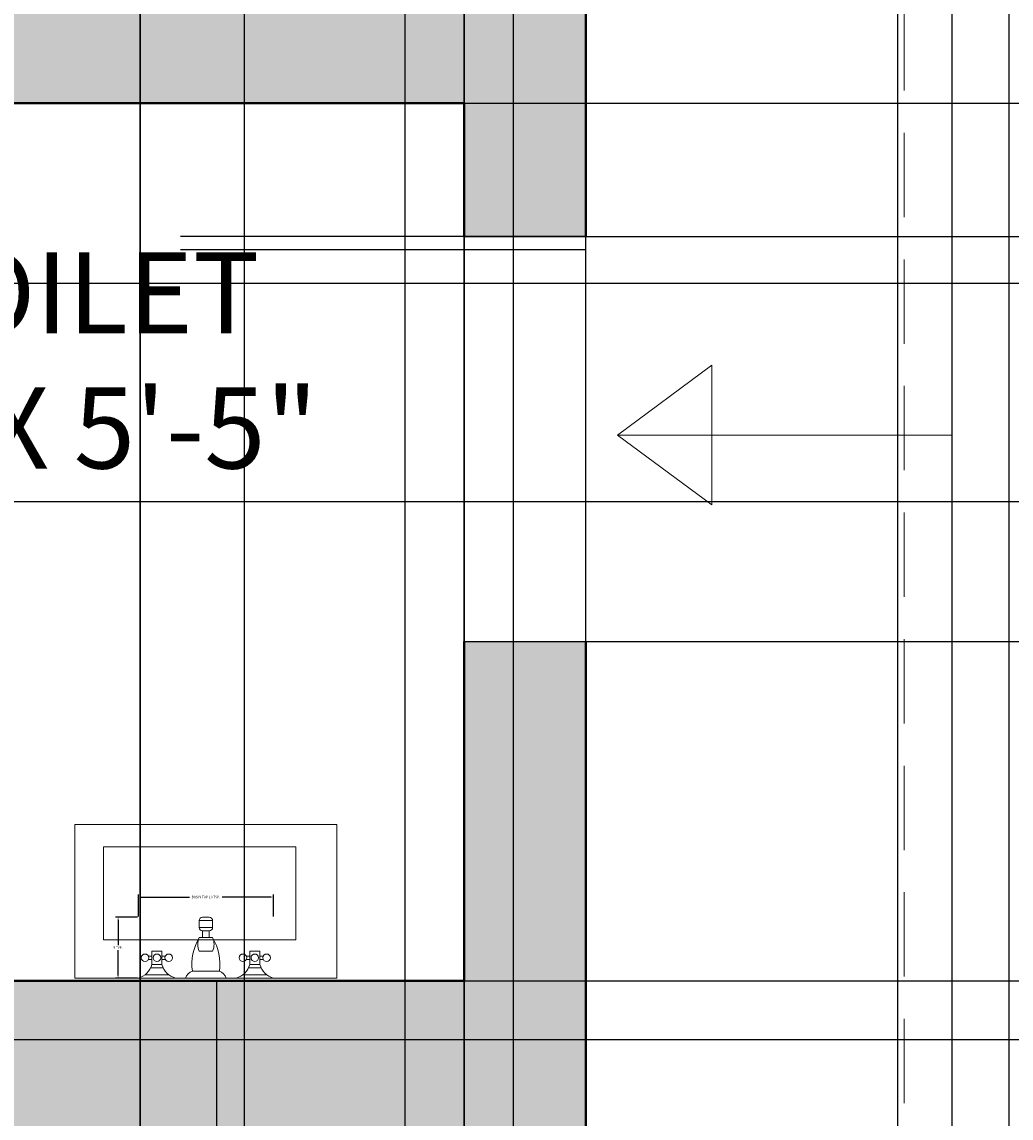
# Model space of a CAD drawing. Units: inches. Extents: x 818 to 1898, y 976 to 2364.
# Tile 55 of 96: x 1673 to 1746, y 1792 to 1873. Entities that reach past the tile are written whole.
import ezdxf

# ---------------------------------------------------------------- set-up
doc = ezdxf.new("R2010")
doc.units = ezdxf.units.IN
doc.header["$LTSCALE"] = 5
doc.header["$MEASUREMENT"] = 0
doc.linetypes.add('HIDDEN', pattern=[0.375, 0.25, -0.125])
for name, color, linetype, lineweight in [('A-ANNO-DIMS', 2, 'Continuous', 18), ('A-ANNO-SYMB', 7, 'Continuous', 18), ('A-AREA-IDEN', 7, 'Continuous', 18), ('A-DOOR', 3, 'Continuous', 25), ('A-FLOR-FIXT', 9, 'Continuous', 18), ('A-FLOR-OVHD', 8, 'HIDDEN', 13), ('A-FLOR-STRS', 7, 'Continuous', 25), ('A-WALL', 7, 'Continuous', 40)]:
    doc.layers.add(name, color=color, linetype=linetype, lineweight=lineweight)
doc.layers.add('A-WALL-PATT', color=251, linetype='Continuous', lineweight=13, true_color=0x636466)
doc.styles.get("Standard").update_dxf_attribs({"font": 'arial.ttf'})
doc.dimstyles.get("Standard").update_dxf_attribs({"dimtxt": 0.18, "dimasz": 0.18, "dimexe": 0.18, "dimexo": 0.0625, "dimgap": 0.09, "dimtad": 0, "dimtih": 1, "dimtoh": 1, "dimdec": 4, "dimzin": 0, "dimdsep": 46, "dimtxsty": 'Standard', "dimcen": 0.09, "dimadec": 0, "dimazin": 0, "dimtfac": 1, "dimtdec": 4, "dimtofl": 0, "dimtmove": 0, "dimatfit": 3, "dimfxl": 1, "dimtolj": 1, "dimtzin": 0, "dimarcsym": 0})

# ---------------------------------------------------------------- blocks, each defined once
blk = doc.blocks.new('Faucet - Bathroom front')
for p, q in [((-0.5, 4.25), (0.5, 4.25)), ((0.5, 3.75), (-0.5, 3.75)), ((-0.25, 3), (-0.25, 3.5)), ((0.25, 3.5), (0.25, 3)), ((-0.5, 3), (0.5, 3)), ((-4, 1.625), (-4.25, 1.625)), ((-3.25, 1.625), (-3, 1.625)), ((0.5, 2), (-0.5, 2)), ((3.25, 1.625), (3, 1.625)), ((4, 1.625), (4.25, 1.625)), ((-4, 1.375), (-4.25, 1.375)), ((-3.25, 1.375), (-3, 1.375)), ((3.25, 1.375), (3, 1.375)), ((4, 1.375), (4.25, 1.375)), ((-5, 0), (-2.25, 0)), ((-4.5087, 0.25), (-2.7408, 0.25)), ((-3.1442, 0.75), (-4.0979, 0.75)), ((-1.5, 0), (1.5, 0)), ((-1, 0.5), (1, 0.5)), ((2.25, 0), (5, 0)), ((2.7413, 0.25), (4.5092, 0.25)), ((4.1058, 0.75), (3.1521, 0.75))]:
    blk.add_line(p, q)
for points in [[(-0.5, 3.75), (-0.5, 4.25)], [(-0.25, 4.5), (0.25, 4.5)], [(0.5, 4.25), (0.5, 3.75)], [(0.25, 3.5), (-0.25, 3.5)]]:
    blk.add_lwpolyline(points)
for points in [[(-4, 1), (-4, 2), (-3.25, 2), (-3.25, 1)], [(3.25, 1), (3.25, 2), (4, 2), (4, 1)]]:
    blk.add_lwpolyline(points, close=True)
for centre in [(-4.5, 1.5), (-3.625, 1.5), (-2.75, 1.5), (2.75, 1.5), (3.625, 1.5), (4.5, 1.5)]:
    blk.add_circle(centre, 0.2795)
for centre, radius, start, end in [((-0.2575, 4.2575), 0.2426, 88.22243, 181.7776), ((0.2575, 4.2575), 0.2426, 358.2224, 91.77757), ((-0.2575, 3.7425), 0.2426, 178.2224, 271.7776), ((0.2575, 3.7425), 0.2426, 268.2224, 1.777565), ((3, 1), 4.0311, 150.2551, 187.125), ((0.6413, 2.5), 1.246, 156.3417, 203.6583), ((-3, 1), 4.0311, 352.875, 29.74488), ((-0.6413, 2.5), 1.246, 336.3417, 23.65835), ((-5.375, 1.375), 1.4252, 285.2551, 344.7449), ((-1.875, 1.375), 1.4252, 195.2551, 254.7449), ((1.875, 1.375), 1.4252, 285.2551, 344.7449), ((5.375, 1.375), 1.4252, 195.2551, 254.7449), ((-0.7962, -0.2038), 0.7327, 106.1502, 163.8498), ((0.7962, -0.2038), 0.7327, 16.1502, 73.84979)]:
    blk.add_arc(centre, radius, start, end)
blk = doc.blocks.new('BASIN-COMPACT')
for points in [[(19.386, 0), (19.386, 11.383), (0, 11.383), (0, 0)], [(16.353, 2.839), (16.353, 9.718), (2.106, 9.718), (2.106, 2.839)]]:
    blk.add_lwpolyline(points, close=True)
blk = doc.blocks.new('ARROW-STEP-UP')
at = {"ltscale": 5}
for p, q in [((0, 5.169), (6.971, 10.338)), ((6.971, 10.338), (6.971, 5.169)), ((24.755, 5.169), (0, 5.169)), ((0, 5.169), (6.971, 0)), ((6.971, 0), (6.971, 5.169))]:
    blk.add_line(p, q, dxfattribs=at)
blk = doc.blocks.new('*D34')
at = {"layer": 'A-ANNO-DIMS', "color": 0, "lineweight": -2, "ltscale": 5, "transparency": 16777216}
for p, q in [((1681.598, 1806.847), (1681.598, 1808.464)), ((1681.778, 1808.284), (1685.382, 1808.284)), ((1691.418, 1808.284), (1687.814, 1808.284)), ((1691.598, 1806.847), (1691.598, 1808.464))]:
    blk.add_line(p, q, dxfattribs=at)
at = {"layer": 'A-ANNO-DIMS', "color": 0, "ltscale": 5, "transparency": 16777216}
for points in [[(1681.778, 1808.314), (1681.778, 1808.254), (1681.598, 1808.284)], [(1691.418, 1808.314), (1691.418, 1808.254), (1691.598, 1808.284)]]:
    blk.add_solid(points, dxfattribs=at)
at = {"layer": 'Defpoints', "color": 0, "ltscale": 5, "transparency": 16777216}
for p in [(1691.598, 1808.284), (1681.598, 1806.784), (1691.598, 1806.784)]:
    blk.add_point(p, dxfattribs=at)
at = {"layer": 'A-ANNO-DIMS', "color": 0, "ltscale": 5, "transparency": 16777216, "insert": (1686.598, 1808.284), "char_height": 0.18, "attachment_point": 5}
blk.add_mtext('\\A1;BASIN TAP 10 TYP.', dxfattribs=at)
blk = doc.blocks.new('*D35')
at = {"layer": 'A-ANNO-DIMS', "color": 0, "lineweight": -2, "ltscale": 5, "transparency": 16777216}
for p, q in [((1681.535, 1806.784), (1679.918, 1806.784)), ((1680.098, 1806.604), (1680.098, 1804.715)), ((1680.098, 1802.462), (1680.098, 1804.352)), ((1681.535, 1802.282), (1679.918, 1802.282))]:
    blk.add_line(p, q, dxfattribs=at)
at = {"layer": 'A-ANNO-DIMS', "color": 0, "ltscale": 5, "transparency": 16777216}
for points in [[(1680.068, 1806.604), (1680.128, 1806.604), (1680.098, 1806.784)], [(1680.068, 1802.462), (1680.128, 1802.462), (1680.098, 1802.282)]]:
    blk.add_solid(points, dxfattribs=at)
at = {"layer": 'Defpoints', "color": 0, "ltscale": 5, "transparency": 16777216}
for p in [(1680.098, 1806.784), (1681.598, 1806.784), (1681.598, 1802.282)]:
    blk.add_point(p, dxfattribs=at)
at = {"layer": 'A-ANNO-DIMS', "color": 0, "ltscale": 5, "transparency": 16777216, "insert": (1680.098, 1804.533), "char_height": 0.18, "attachment_point": 5}
blk.add_mtext('\\A1;5 TYP.', dxfattribs=at)
blk = doc.blocks.new('*D71')
at = {"layer": 'A-ANNO-DIMS', "color": 0, "lineweight": -2, "ltscale": 5, "transparency": 16777216}
for p, q in [((1714.788, 2053.078), (1897.916, 2053.078)), ((1897.736, 2052.898), (1897.736, 1699.76)), ((1897.736, 1346.258), (1897.736, 1699.396)), ((1714.788, 1346.078), (1897.916, 1346.078))]:
    blk.add_line(p, q, dxfattribs=at)
at = {"layer": 'A-ANNO-DIMS', "color": 0, "ltscale": 5, "transparency": 16777216}
for points in [[(1897.706, 2052.898), (1897.766, 2052.898), (1897.736, 2053.078)], [(1897.706, 1346.258), (1897.766, 1346.258), (1897.736, 1346.078)]]:
    blk.add_solid(points, dxfattribs=at)
at = {"layer": 'Defpoints', "color": 0, "ltscale": 5, "transparency": 16777216}
for p in [(1714.725, 2053.078), (1897.736, 2053.078), (1714.725, 1346.078)]:
    blk.add_point(p, dxfattribs=at)
at = {"layer": 'A-ANNO-DIMS', "color": 0, "ltscale": 5, "transparency": 16777216, "insert": (1897.736, 1699.578), "char_height": 0.18, "attachment_point": 5}
blk.add_mtext('\\A1;707', dxfattribs=at)
blk = doc.blocks.new('*D76')
at = {"layer": 'A-ANNO-DIMS', "color": 0, "lineweight": -2, "ltscale": 5, "transparency": 16777216}
for p, q in [((1705.788, 1857.212), (1897.916, 1857.212)), ((1897.736, 1857.032), (1897.736, 1842.394)), ((1897.736, 1827.392), (1897.736, 1842.031)), ((1705.788, 1827.212), (1897.916, 1827.212))]:
    blk.add_line(p, q, dxfattribs=at)
at = {"layer": 'A-ANNO-DIMS', "color": 0, "ltscale": 5, "transparency": 16777216}
for points in [[(1897.706, 1857.032), (1897.766, 1857.032), (1897.736, 1857.212)], [(1897.706, 1827.392), (1897.766, 1827.392), (1897.736, 1827.212)]]:
    blk.add_solid(points, dxfattribs=at)
at = {"layer": 'Defpoints', "color": 0, "ltscale": 5, "transparency": 16777216}
for p in [(1705.725, 1857.212), (1897.736, 1857.212), (1705.725, 1827.212)]:
    blk.add_point(p, dxfattribs=at)
at = {"layer": 'A-ANNO-DIMS', "color": 0, "ltscale": 5, "transparency": 16777216, "insert": (1897.736, 1842.212), "char_height": 0.18, "attachment_point": 5}
blk.add_mtext('\\A1;30', dxfattribs=at)
blk = doc.blocks.new('*D85')
at = {"layer": 'A-ANNO-DIMS', "color": 0, "lineweight": -2, "ltscale": 5, "transparency": 16777216}
for p, q in [((1258.788, 2053.078), (1897.916, 2053.078)), ((1897.736, 2052.898), (1897.736, 1876.76)), ((1897.736, 1700.258), (1897.736, 1876.396)), ((1258.788, 1700.078), (1897.916, 1700.078))]:
    blk.add_line(p, q, dxfattribs=at)
at = {"layer": 'A-ANNO-DIMS', "color": 0, "ltscale": 5, "transparency": 16777216}
for points in [[(1897.706, 2052.898), (1897.766, 2052.898), (1897.736, 2053.078)], [(1897.706, 1700.258), (1897.766, 1700.258), (1897.736, 1700.078)]]:
    blk.add_solid(points, dxfattribs=at)
at = {"layer": 'Defpoints', "color": 0, "ltscale": 5, "transparency": 16777216}
for p in [(1258.725, 2053.078), (1897.736, 2053.078), (1258.725, 1700.078)]:
    blk.add_point(p, dxfattribs=at)
at = {"layer": 'A-ANNO-DIMS', "color": 0, "ltscale": 5, "transparency": 16777216, "insert": (1897.736, 1876.578), "char_height": 0.18, "attachment_point": 5}
blk.add_mtext('\\A1;353', dxfattribs=at)
blk = doc.blocks.new('*D103')
at = {"layer": 'A-ANNO-DIMS', "color": 0, "lineweight": -2, "ltscale": 5, "transparency": 16777216}
for p, q in [((1626.575, 1071.118), (1626.575, 2363.873)), ((1626.755, 2363.693), (1657.699, 2363.693)), ((1689.291, 2363.693), (1658.348, 2363.693)), ((1689.471, 1071.118), (1689.471, 2363.873))]:
    blk.add_line(p, q, dxfattribs=at)
at = {"layer": 'A-ANNO-DIMS', "color": 0, "ltscale": 5, "transparency": 16777216}
for points in [[(1626.755, 2363.723), (1626.755, 2363.663), (1626.575, 2363.693)], [(1689.291, 2363.723), (1689.291, 2363.663), (1689.471, 2363.693)]]:
    blk.add_solid(points, dxfattribs=at)
at = {"layer": 'Defpoints', "color": 0, "ltscale": 5, "transparency": 16777216}
for p in [(1689.471, 2363.693), (1626.575, 1071.055), (1689.471, 1071.055)]:
    blk.add_point(p, dxfattribs=at)
at = {"layer": 'A-ANNO-DIMS', "color": 0, "ltscale": 5, "transparency": 16777216, "insert": (1658.023, 2363.693), "char_height": 0.18, "attachment_point": 5}
blk.add_mtext('\\A1;62.9', dxfattribs=at)
blk = doc.blocks.new('*D104')
at = {"layer": 'A-ANNO-DIMS', "color": 0, "lineweight": -2, "ltscale": 5, "transparency": 16777216}
for p, q in [((1689.471, 1071.118), (1689.471, 2363.873)), ((1689.651, 2363.693), (1717.401, 2363.693)), ((1745.903, 2363.693), (1718.154, 2363.693)), ((1746.083, 1071.118), (1746.083, 2363.873))]:
    blk.add_line(p, q, dxfattribs=at)
at = {"layer": 'A-ANNO-DIMS', "color": 0, "ltscale": 5, "transparency": 16777216}
for points in [[(1689.651, 2363.723), (1689.651, 2363.663), (1689.471, 2363.693)], [(1745.903, 2363.723), (1745.903, 2363.663), (1746.083, 2363.693)]]:
    blk.add_solid(points, dxfattribs=at)
at = {"layer": 'Defpoints', "color": 0, "ltscale": 5, "transparency": 16777216}
for p in [(1746.083, 2363.693), (1689.471, 1071.055), (1746.083, 1071.055)]:
    blk.add_point(p, dxfattribs=at)
at = {"layer": 'A-ANNO-DIMS', "color": 0, "ltscale": 5, "transparency": 16777216, "insert": (1717.777, 2363.693), "char_height": 0.18, "attachment_point": 5}
blk.add_mtext('\\A1;56.61', dxfattribs=at)
blk = doc.blocks.new('*D120')
at = {"layer": 'A-ANNO-DIMS', "color": 0, "lineweight": -2, "ltscale": 5, "transparency": 16777216}
for p, q in [((1766.29, 1797.717), (818.026, 1797.717)), ((818.206, 1797.537), (818.206, 1757.534)), ((818.206, 1717.167), (818.206, 1757.17)), ((1766.29, 1716.987), (818.026, 1716.987))]:
    blk.add_line(p, q, dxfattribs=at)
at = {"layer": 'A-ANNO-DIMS', "color": 0, "ltscale": 5, "transparency": 16777216}
for points in [[(818.176, 1797.537), (818.236, 1797.537), (818.206, 1797.717)], [(818.176, 1717.167), (818.236, 1717.167), (818.206, 1716.987)]]:
    blk.add_solid(points, dxfattribs=at)
at = {"layer": 'Defpoints', "color": 0, "ltscale": 5, "transparency": 16777216}
for p in [(818.206, 1797.717), (1766.352, 1797.717), (1766.352, 1716.987)]:
    blk.add_point(p, dxfattribs=at)
at = {"layer": 'A-ANNO-DIMS', "color": 0, "ltscale": 5, "transparency": 16777216, "insert": (818.206, 1757.352), "char_height": 0.18, "attachment_point": 5}
blk.add_mtext('\\A1;80.73', dxfattribs=at)
blk = doc.blocks.new('*D121')
at = {"layer": 'A-ANNO-DIMS', "color": 0, "lineweight": -2, "ltscale": 5, "transparency": 16777216}
for p, q in [((1766.29, 1884.203), (818.026, 1884.203)), ((818.206, 1884.023), (818.206, 1841.142)), ((818.206, 1797.897), (818.206, 1840.778)), ((1766.29, 1797.717), (818.026, 1797.717))]:
    blk.add_line(p, q, dxfattribs=at)
at = {"layer": 'A-ANNO-DIMS', "color": 0, "ltscale": 5, "transparency": 16777216}
for points in [[(818.176, 1884.023), (818.236, 1884.023), (818.206, 1884.203)], [(818.176, 1797.897), (818.236, 1797.897), (818.206, 1797.717)]]:
    blk.add_solid(points, dxfattribs=at)
at = {"layer": 'Defpoints', "color": 0, "ltscale": 5, "transparency": 16777216}
for p in [(818.206, 1884.203), (1766.352, 1884.203), (1766.352, 1797.717)]:
    blk.add_point(p, dxfattribs=at)
at = {"layer": 'A-ANNO-DIMS', "color": 0, "ltscale": 5, "transparency": 16777216, "insert": (818.206, 1840.96), "char_height": 0.18, "attachment_point": 5}
blk.add_mtext('\\A1;86.49', dxfattribs=at)
blk = doc.blocks.new('*D154')
at = {"layer": 'A-ANNO-DIMS', "color": 0, "lineweight": -2, "ltscale": 5, "transparency": 16777216}
for p, q in [((1701.369, 1290.141), (1701.369, 2363.873)), ((1701.549, 2363.693), (1705.22, 2363.693)), ((1709.189, 2363.693), (1705.518, 2363.693)), ((1709.369, 1298.141), (1709.369, 2363.873))]:
    blk.add_line(p, q, dxfattribs=at)
at = {"layer": 'A-ANNO-DIMS', "color": 0, "ltscale": 5, "transparency": 16777216}
for points in [[(1701.549, 2363.723), (1701.549, 2363.663), (1701.369, 2363.693)], [(1709.189, 2363.723), (1709.189, 2363.663), (1709.369, 2363.693)]]:
    blk.add_solid(points, dxfattribs=at)
at = {"layer": 'Defpoints', "color": 0, "ltscale": 5, "transparency": 16777216}
for p in [(1709.369, 2363.693), (1709.369, 1298.078), (1701.369, 1290.078)]:
    blk.add_point(p, dxfattribs=at)
at = {"layer": 'A-ANNO-DIMS', "color": 0, "ltscale": 5, "transparency": 16777216, "insert": (1705.369, 2363.693), "char_height": 0.18, "attachment_point": 5}
blk.add_mtext('\\A1;8', dxfattribs=at)
blk = doc.blocks.new('*D186')
at = {"layer": 'A-ANNO-DIMS', "color": 0, "lineweight": -2, "ltscale": 5, "transparency": 16777216}
for p, q in [((1714.725, 1549.141), (1714.725, 2363.873)), ((1714.905, 2363.693), (1725.818, 2363.693)), ((1737.661, 2363.693), (1726.748, 2363.693)), ((1737.841, 1549.141), (1737.841, 2363.873))]:
    blk.add_line(p, q, dxfattribs=at)
at = {"layer": 'A-ANNO-DIMS', "color": 0, "ltscale": 5, "transparency": 16777216}
for points in [[(1714.905, 2363.723), (1714.905, 2363.663), (1714.725, 2363.693)], [(1737.661, 2363.723), (1737.661, 2363.663), (1737.841, 2363.693)]]:
    blk.add_solid(points, dxfattribs=at)
at = {"layer": 'Defpoints', "color": 0, "ltscale": 5, "transparency": 16777216}
for p in [(1737.841, 2363.693), (1714.725, 1549.078), (1737.841, 1549.078)]:
    blk.add_point(p, dxfattribs=at)
at = {"layer": 'A-ANNO-DIMS', "color": 0, "ltscale": 5, "transparency": 16777216, "insert": (1726.283, 2363.693), "char_height": 0.18, "attachment_point": 5}
blk.add_mtext('\\A1;23.116', dxfattribs=at)
blk = doc.blocks.new('*D195')
at = {"layer": 'A-ANNO-DIMS', "color": 0, "lineweight": -2, "ltscale": 5, "transparency": 16777216}
for p, q in [((1681.725, 1379.141), (1681.725, 2363.873)), ((1681.905, 2363.693), (1693.505, 2363.693)), ((1705.545, 2363.693), (1693.945, 2363.693)), ((1705.725, 1355.141), (1705.725, 2363.873))]:
    blk.add_line(p, q, dxfattribs=at)
at = {"layer": 'A-ANNO-DIMS', "color": 0, "ltscale": 5, "transparency": 16777216}
for points in [[(1681.905, 2363.723), (1681.905, 2363.663), (1681.725, 2363.693)], [(1705.545, 2363.723), (1705.545, 2363.663), (1705.725, 2363.693)]]:
    blk.add_solid(points, dxfattribs=at)
at = {"layer": 'Defpoints', "color": 0, "ltscale": 5, "transparency": 16777216}
for p in [(1705.725, 2363.693), (1681.725, 1379.078), (1705.725, 1355.078)]:
    blk.add_point(p, dxfattribs=at)
at = {"layer": 'A-ANNO-DIMS', "color": 0, "ltscale": 5, "transparency": 16777216, "insert": (1693.725, 2363.693), "char_height": 0.18, "attachment_point": 5}
blk.add_mtext('\\A1;24', dxfattribs=at)
blk = doc.blocks.new('*D204')
at = {"layer": 'A-ANNO-DIMS', "color": 0, "lineweight": -2, "ltscale": 5, "transparency": 16777216}
for p, q in [((1714.788, 2053.078), (1897.916, 2053.078)), ((1897.736, 2052.898), (1897.736, 1960.26)), ((1897.736, 1867.258), (1897.736, 1959.896)), ((1705.788, 1867.078), (1897.916, 1867.078))]:
    blk.add_line(p, q, dxfattribs=at)
at = {"layer": 'A-ANNO-DIMS', "color": 0, "ltscale": 5, "transparency": 16777216}
for points in [[(1897.706, 2052.898), (1897.766, 2052.898), (1897.736, 2053.078)], [(1897.706, 1867.258), (1897.766, 1867.258), (1897.736, 1867.078)]]:
    blk.add_solid(points, dxfattribs=at)
at = {"layer": 'Defpoints', "color": 0, "ltscale": 5, "transparency": 16777216}
for p in [(1714.725, 2053.078), (1897.736, 2053.078), (1705.725, 1867.078)]:
    blk.add_point(p, dxfattribs=at)
at = {"layer": 'A-ANNO-DIMS', "color": 0, "ltscale": 5, "transparency": 16777216, "insert": (1897.736, 1960.078), "char_height": 0.18, "attachment_point": 5}
blk.add_mtext('\\A1;186', dxfattribs=at)
blk = doc.blocks.new('*D212')
at = {"layer": 'A-ANNO-DIMS', "color": 0, "lineweight": -2, "ltscale": 5, "transparency": 16777216}
for p, q in [((1681.725, 1900.016), (1681.725, 975.663)), ((1705.725, 1876.016), (1705.725, 975.663)), ((1681.905, 975.843), (1693.505, 975.843)), ((1705.545, 975.843), (1693.945, 975.843))]:
    blk.add_line(p, q, dxfattribs=at)
at = {"layer": 'A-ANNO-DIMS', "color": 0, "ltscale": 5, "transparency": 16777216}
for points in [[(1681.905, 975.873), (1681.905, 975.813), (1681.725, 975.843)], [(1705.545, 975.873), (1705.545, 975.813), (1705.725, 975.843)]]:
    blk.add_solid(points, dxfattribs=at)
at = {"layer": 'Defpoints', "color": 0, "ltscale": 5, "transparency": 16777216}
for p in [(1681.725, 1900.078), (1705.725, 1876.078), (1705.725, 975.843)]:
    blk.add_point(p, dxfattribs=at)
at = {"layer": 'A-ANNO-DIMS', "color": 0, "ltscale": 5, "transparency": 16777216, "insert": (1693.725, 975.843), "char_height": 0.18, "attachment_point": 5}
blk.add_mtext('\\A1;24', dxfattribs=at)
blk = doc.blocks.new('*D218')
at = {"layer": 'A-ANNO-DIMS', "color": 0, "lineweight": -2, "ltscale": 5, "transparency": 16777216}
for p, q in [((1705.788, 1827.212), (1897.916, 1827.212)), ((1897.736, 1827.032), (1897.736, 1814.827)), ((1897.736, 1802.258), (1897.736, 1814.463)), ((1705.788, 1802.078), (1897.916, 1802.078))]:
    blk.add_line(p, q, dxfattribs=at)
at = {"layer": 'A-ANNO-DIMS', "color": 0, "ltscale": 5, "transparency": 16777216}
for points in [[(1897.706, 1827.032), (1897.766, 1827.032), (1897.736, 1827.212)], [(1897.706, 1802.258), (1897.766, 1802.258), (1897.736, 1802.078)]]:
    blk.add_solid(points, dxfattribs=at)
at = {"layer": 'Defpoints', "color": 0, "ltscale": 5, "transparency": 16777216}
for p in [(1705.725, 1827.212), (1897.736, 1827.212), (1705.725, 1802.078)]:
    blk.add_point(p, dxfattribs=at)
at = {"layer": 'A-ANNO-DIMS', "color": 0, "ltscale": 5, "transparency": 16777216, "insert": (1897.736, 1814.645), "char_height": 0.18, "attachment_point": 5}
blk.add_mtext('\\A1;25.134', dxfattribs=at)
blk = doc.blocks.new('*D225')
at = {"layer": 'A-ANNO-DIMS', "color": 0, "lineweight": -2, "ltscale": 5, "transparency": 16777216}
for p, q in [((1532.655, 1867.078), (1897.916, 1867.078)), ((1897.736, 1866.898), (1897.736, 1852.512)), ((1897.736, 1837.762), (1897.736, 1852.148)), ((1532.655, 1837.582), (1897.916, 1837.582))]:
    blk.add_line(p, q, dxfattribs=at)
at = {"layer": 'A-ANNO-DIMS', "color": 0, "ltscale": 5, "transparency": 16777216}
for points in [[(1897.706, 1866.898), (1897.766, 1866.898), (1897.736, 1867.078)], [(1897.706, 1837.762), (1897.766, 1837.762), (1897.736, 1837.582)]]:
    blk.add_solid(points, dxfattribs=at)
at = {"layer": 'Defpoints', "color": 0, "ltscale": 5, "transparency": 16777216}
for p in [(1532.593, 1867.078), (1897.736, 1867.078), (1532.593, 1837.582)]:
    blk.add_point(p, dxfattribs=at)
at = {"layer": 'A-ANNO-DIMS', "color": 0, "ltscale": 5, "transparency": 16777216, "insert": (1897.736, 1852.33), "char_height": 0.18, "attachment_point": 5}
blk.add_mtext('\\A1;29.496', dxfattribs=at)
blk = doc.blocks.new('*D228')
at = {"layer": 'A-ANNO-DIMS', "color": 0, "lineweight": -2, "ltscale": 5, "transparency": 16777216}
for p, q in [((1687.394, 1802.016), (1687.394, 975.663)), ((1705.725, 1802.016), (1705.725, 975.663)), ((1687.574, 975.843), (1696.174, 975.843)), ((1705.545, 975.843), (1696.945, 975.843))]:
    blk.add_line(p, q, dxfattribs=at)
at = {"layer": 'A-ANNO-DIMS', "color": 0, "ltscale": 5, "transparency": 16777216}
for points in [[(1687.574, 975.873), (1687.574, 975.813), (1687.394, 975.843)], [(1705.545, 975.873), (1705.545, 975.813), (1705.725, 975.843)]]:
    blk.add_solid(points, dxfattribs=at)
at = {"layer": 'Defpoints', "color": 0, "ltscale": 5, "transparency": 16777216}
for p in [(1687.394, 1802.078), (1705.725, 1802.078), (1705.725, 975.843)]:
    blk.add_point(p, dxfattribs=at)
at = {"layer": 'A-ANNO-DIMS', "color": 0, "ltscale": 5, "transparency": 16777216, "insert": (1696.56, 975.843), "char_height": 0.18, "attachment_point": 5}
blk.add_mtext('\\A1;18.33', dxfattribs=at)
blk = doc.blocks.new('*D268')
at = {"layer": 'A-ANNO-DIMS', "color": 0, "lineweight": -2, "ltscale": 5, "transparency": 16777216}
for p, q in [((1741.903, 1890.29), (1897.916, 1890.29)), ((1897.736, 1890.11), (1897.736, 1788.866)), ((1897.736, 1687.258), (1897.736, 1788.502)), ((1741.903, 1687.078), (1897.916, 1687.078))]:
    blk.add_line(p, q, dxfattribs=at)
at = {"layer": 'A-ANNO-DIMS', "color": 0, "ltscale": 5, "transparency": 16777216}
for points in [[(1897.706, 1890.11), (1897.766, 1890.11), (1897.736, 1890.29)], [(1897.706, 1687.258), (1897.766, 1687.258), (1897.736, 1687.078)]]:
    blk.add_solid(points, dxfattribs=at)
at = {"layer": 'Defpoints', "color": 0, "ltscale": 5, "transparency": 16777216}
for p in [(1741.841, 1890.29), (1897.736, 1890.29), (1741.841, 1687.078)]:
    blk.add_point(p, dxfattribs=at)
at = {"layer": 'A-ANNO-DIMS', "color": 0, "ltscale": 5, "transparency": 16777216, "insert": (1897.736, 1788.684), "char_height": 0.18, "attachment_point": 5}
blk.add_mtext('\\A1;203.2', dxfattribs=at)
blk = doc.blocks.new('*D275')
at = {"layer": 'A-ANNO-DIMS', "color": 0, "lineweight": -2, "ltscale": 5, "transparency": 16777216}
for p, q in [((1377.842, 1897.866), (1897.916, 1897.866)), ((1897.736, 1897.686), (1897.736, 1875.988)), ((1897.736, 1853.93), (1897.736, 1875.628)), ((1377.842, 1853.75), (1897.916, 1853.75))]:
    blk.add_line(p, q, dxfattribs=at)
at = {"layer": 'A-ANNO-DIMS', "color": 0, "ltscale": 5, "transparency": 16777216}
for points in [[(1897.706, 1897.686), (1897.766, 1897.686), (1897.736, 1897.866)], [(1897.706, 1853.93), (1897.766, 1853.93), (1897.736, 1853.75)]]:
    blk.add_solid(points, dxfattribs=at)
at = {"layer": 'Defpoints', "color": 0, "ltscale": 5, "transparency": 16777216}
for p in [(1377.779, 1897.866), (1897.736, 1897.866), (1377.779, 1853.75)]:
    blk.add_point(p, dxfattribs=at)
at = {"layer": 'A-ANNO-DIMS', "color": 0, "ltscale": 5, "transparency": 16777216, "insert": (1897.736, 1875.808), "char_height": 0.18, "attachment_point": 5}
blk.add_mtext('\\A1;44.12', dxfattribs=at)
blk = doc.blocks.new('*D282')
at = {"layer": 'A-ANNO-DIMS', "color": 0, "lineweight": -2, "ltscale": 5, "transparency": 16777216}
for p, q in [((1422.083, 2081.188), (1897.916, 2081.188)), ((1897.736, 2081.008), (1897.736, 1884.315)), ((1897.736, 1687.258), (1897.736, 1883.951)), ((1463.788, 1687.078), (1897.916, 1687.078))]:
    blk.add_line(p, q, dxfattribs=at)
at = {"layer": 'A-ANNO-DIMS', "color": 0, "ltscale": 5, "transparency": 16777216}
for points in [[(1897.706, 2081.008), (1897.766, 2081.008), (1897.736, 2081.188)], [(1897.706, 1687.258), (1897.766, 1687.258), (1897.736, 1687.078)]]:
    blk.add_solid(points, dxfattribs=at)
at = {"layer": 'Defpoints', "color": 0, "ltscale": 5, "transparency": 16777216}
for p in [(1422.02, 2081.188), (1897.736, 2081.188), (1463.725, 1687.078)]:
    blk.add_point(p, dxfattribs=at)
at = {"layer": 'A-ANNO-DIMS', "color": 0, "ltscale": 5, "transparency": 16777216, "insert": (1897.736, 1884.133), "char_height": 0.18, "attachment_point": 5}
blk.add_mtext('\\A1;394.1', dxfattribs=at)

msp = doc.modelspace()

# ---------------------------------------------------------------- hatches: boundary and pattern name
at = {"layer": 'A-WALL-PATT', "ltscale": 5}
h = msp.add_hatch(color=256, dxfattribs=at)
h.dxf.hatch_style = 1
h.paths.add_polyline_path([(1267.7252, 1928.9218), (1258.7251, 1928.9218), (1258.7251, 1913.6401), (1250.3029, 1913.6401), (1250.3029, 1878.3919), (1258.7251, 1878.3919), (1258.7251, 1862.9652), (1267.7252, 1862.9652)])
h.paths.add_polyline_path([(1267.7252, 1814.9652), (1258.7251, 1814.9652), (1258.7251, 1755.3321), (1267.7252, 1755.3321)])
h.paths.add_polyline_path([(1463.7251, 1696.0782), (1267.7252, 1696.0782), (1267.7252, 1707.3321), (1258.7251, 1707.3321), (1258.7251, 1700.0782), (1251.9333, 1700.0782), (1251.9333, 1687.0782), (1463.7251, 1687.0782)])
h.paths.add_polyline_path([(1714.7251, 1717.3178), (1705.7251, 1717.3178), (1705.7251, 1696.0782), (1599.7252, 1696.0782), (1599.7252, 1790.0782), (1705.7251, 1790.0782), (1705.7251, 1785.6125), (1714.7251, 1785.6125), (1714.7251, 1827.2125), (1705.7251, 1827.2125), (1705.7251, 1802.0782), (1599.7252, 1802.0782), (1599.7252, 1867.0782), (1705.7251, 1867.0782), (1705.7251, 1857.2125), (1714.7251, 1857.2125), (1714.7251, 1930.0316), (1741.8409, 1930.0316), (1741.8409, 1935.0316), (1714.7251, 1935.0316), (1714.7251, 1957.0338), (1741.8409, 1957.0338), (1741.8409, 1962.0338), (1714.7251, 1962.0338), (1705.7251, 1962.0338), (1705.7251, 1948.0782), (1599.7252, 1948.0782), (1599.7252, 1981.0782), (1590.7252, 1981.0782), (1590.7252, 1941.0782), (1620.7252, 1941.0782), (1705.7251, 1941.0782), (1705.7251, 1876.0782), (1599.7252, 1876.0782), (1599.7252, 1911.0782), (1590.7252, 1911.0782), (1590.7252, 1876.0782), (1429.2252, 1876.0782), (1429.2252, 1867.0782), (1511.7252, 1867.0782), (1528.593, 1867.0782), (1595.7252, 1867.0782), (1595.7252, 1773.0782), (1520.7252, 1773.0782), (1520.7252, 1837.5823), (1532.593, 1837.5823), (1532.593, 1867.0782), (1528.593, 1867.0782), (1528.593, 1841.5823), (1511.7252, 1841.5823), (1511.7252, 1744.9714), (1520.7252, 1744.9714), (1520.7252, 1761.0782), (1595.7252, 1761.0782), (1595.7252, 1696.0782), (1520.7252, 1696.0782), (1520.7252, 1716.0454), (1511.7252, 1716.0454), (1511.7252, 1696.0782), (1511.7252, 1687.0782), (1714.7251, 1687.0782)])
h.paths.add_polyline_path([(1714.7251, 2053.0782), (1714.7251, 2081.1881), (1709.7252, 2081.1881), (1709.7252, 2053.0782), (1681.6446, 2053.0782), (1681.6446, 2081.1881), (1676.6446, 2081.1881), (1676.6446, 2053.0782), (1538.5155, 2053.0782), (1538.5155, 2044.0782), (1590.7252, 2044.0782), (1590.7252, 2011.0782), (1599.7252, 2011.0782), (1599.7252, 2044.0782), (1705.7251, 2044.0782), (1705.7251, 2014.5114), (1714.7251, 2014.5114)])
h.paths.add_polyline_path([(1485.1216, 2053.0782), (1422.02, 2053.0782), (1422.02, 2081.1881), (1413.02, 2081.1881), (1413.02, 2053.0782), (1399.6356, 2053.0782), (1399.6356, 2081.1881), (1390.6356, 2081.1881), (1390.6356, 2053.0782), (1388.0315, 2053.0782), (1388.0315, 2044.0782), (1416.2743, 2044.0782), (1485.1216, 2044.0782)])
h.paths.add_polyline_path([(1330.305, 2053.0782), (1258.7251, 2053.0782), (1258.7251, 2019.2871), (1267.7252, 2019.2871), (1267.7252, 2044.0782), (1330.305, 2044.0782)])
h.paths.add_polyline_path([(1258.7251, 2053.0782), (1214.6577, 2053.0782), (1214.6577, 2044.0782), (1258.7251, 2044.0782)])
h.paths.add_polyline_path([(1214.6577, 2053.0782), (1180.349, 2053.0782), (1180.349, 2044.0782), (1214.6577, 2044.0782)])
h.paths.add_polyline_path([(1714.7251, 1639.5782), (1741.8409, 1639.5782), (1741.8409, 1643.5782), (1714.7251, 1643.5782), (1714.7251, 1649.9029), (1705.7251, 1649.9029), (1705.7251, 1600.0782), (1477.7252, 1600.0782), (1477.7252, 1591.0782), (1520.7252, 1591.0782), (1616.7252, 1591.0782), (1616.7252, 1416.6857), (1622.7252, 1416.6857), (1622.7252, 1463.0782), (1624.7252, 1463.0782), (1624.7252, 1467.0782), (1622.7252, 1467.0782), (1622.7252, 1591.0782), (1705.7251, 1591.0782), (1705.7251, 1545.0782), (1714.7251, 1545.0782), (1741.8409, 1545.0782), (1741.8409, 1549.0782), (1714.7251, 1549.0782), (1714.7251, 1593.9175), (1737.8409, 1593.9175), (1737.8409, 1597.9175), (1714.7251, 1597.9175)])
h.paths.add_polyline_path([(1674.9024, 2060.7419), (1714.7045, 2060.7419), (1714.7045, 2073.1061), (1674.9024, 2073.1061)], flags=25)
h.paths.add_polyline_path([(1394.5468, 2061.6618), (1422.2344, 2061.6618), (1422.2344, 2074.0261), (1394.5468, 2074.0261)], flags=24)

# ---------------------------------------------------------------- linework, layer by layer
at = {"layer": 'A-DOOR'}
for p, q in [((1714.7251, 1857.2125), (1684.7252, 1857.2125)), ((1705.7251, 1857.2125), (1714.7251, 1857.2125)), ((1714.7251, 1856.2125), (1684.7252, 1856.2125)), ((1705.7251, 1827.2125), (1714.7251, 1827.2125))]:
    msp.add_line(p, q, dxfattribs=at)
at = {"layer": 'A-FLOR-OVHD', "ltscale": 5}
msp.add_line((1738.3002, 1883.6351), (1738.3002, 1692.5441), dxfattribs=at)
at = {"layer": 'A-FLOR-STRS'}
msp.add_line((1741.8409, 1890.2903), (1741.8409, 1759.6099), dxfattribs=at)
at = {"layer": 'A-WALL'}
for p, q in [((1714.7251, 1930.0316), (1714.7251, 1857.2125)), ((1599.7252, 1867.0782), (1705.7251, 1867.0782)), ((1705.7251, 1867.0782), (1705.7251, 1857.2125)), ((1705.7251, 1827.2125), (1705.7251, 1802.0782)), ((1714.7251, 1827.2125), (1714.7251, 1785.6125)), ((1599.7252, 1802.0782), (1705.7251, 1802.0782))]:
    msp.add_line(p, q, dxfattribs=at)

# ---------------------------------------------------------------- block references
at = {"layer": 'A-ANNO-SYMB'}
msp.add_blockref('ARROW-STEP-UP', (1717.086, 1837.331), dxfattribs=at)
at = {"layer": 'A-FLOR-FIXT'}
for name, p in [('BASIN-COMPACT', (1676.9048, 1802.2817)), ('Faucet - Bathroom front', (1686.5978, 1802.282))]:
    msp.add_blockref(name, p, dxfattribs=at)

# ---------------------------------------------------------------- texts
at = {"layer": 'A-AREA-IDEN', "ltscale": 5, "insert": (1645.8362, 1856.0216), "char_height": 6, "attachment_point": 1}
msp.add_mtext_dynamic_manual_height_columns('SER.TOILET\\P8\'-10" X 5\'-5"', width=118.992422, gutter_width=1, heights=[0], dxfattribs=at)

# ---------------------------------------------------------------- dimensions: what is measured, and where the dimension line sits
at = {"layer": 'A-ANNO-DIMS', "ltscale": 5}
for base, p1, p2, override, picture, middle in [((1689.4714, 2363.6929), (1626.5748, 1071.0552), (1689.4714, 1071.0552), {"dimdec": 1, "dimlfac": 1, "dimrnd": 0, "dimzin": 0, "dimdsep": 46, "dimlunit": 2}, '*D103', (1658.0231, 2363.6929)), ((1705.7251, 2363.6929), (1681.7251, 1379.0782), (1705.7251, 1355.0782), {"dimdec": 0, "dimlfac": 1, "dimrnd": 0, "dimzin": 0, "dimdsep": 46, "dimlunit": 2}, '*D195', (1693.7251, 2363.6929)), ((1746.0831, 2363.6929), (1689.4714, 1071.0552), (1746.0831, 1071.0552), {"dimdec": 2, "dimlfac": 1, "dimrnd": 0, "dimzin": 0, "dimdsep": 46, "dimlunit": 2}, '*D104', (1717.7772, 2363.6929)), ((1709.3688, 2363.6929), (1701.3688, 1290.0782), (1709.3688, 1298.0782), {"dimdec": 0, "dimlfac": 1, "dimrnd": 0, "dimzin": 0, "dimdsep": 46, "dimlunit": 2}, '*D154', (1705.3688, 2363.6929)), ((1737.8409, 2363.6929), (1714.7251, 1549.0782), (1737.8409, 1549.0782), {"dimdec": 3, "dimlfac": 1, "dimrnd": 0, "dimzin": 0, "dimdsep": 46, "dimlunit": 2}, '*D186', (1726.283, 2363.6929)), ((1705.7251, 975.8433), (1681.7251, 1900.0782), (1705.7251, 1876.0782), {"dimdec": 0, "dimlfac": 1, "dimrnd": 0, "dimzin": 0, "dimdsep": 46, "dimlunit": 2}, '*D212', (1693.7251, 975.8433)), ((1705.7251, 975.8433), (1687.394, 1802.0782), (1705.7251, 1802.0782), {"dimdec": 2, "dimlfac": 1, "dimrnd": 0, "dimzin": 0, "dimdsep": 46, "dimlunit": 2}, '*D228', (1696.5596, 975.8433))]:
    dim = msp.add_linear_dim(base=base, p1=p1, p2=p2, dimstyle='Standard', override=override, dxfattribs=at)
    dim.commit()
    dim.dimension.update_dxf_attribs({"geometry": picture, "text_midpoint": middle})
for base, p1, p2, override, picture, middle in [((1897.736, 2081.1881), (1463.7251, 1687.0782), (1422.02, 2081.1881), {"dimdec": 1, "dimlfac": 1, "dimrnd": 0, "dimzin": 0, "dimdsep": 46, "dimlunit": 2}, '*D282', (1897.736, 1884.1332)), ((1897.736, 2053.0782), (1258.7251, 1700.0782), (1258.7251, 2053.0782), {"dimdec": 0, "dimlfac": 1, "dimrnd": 0, "dimzin": 0, "dimdsep": 46, "dimlunit": 2}, '*D85', (1897.736, 1876.5782)), ((1897.736, 2053.0782), (1705.7251, 1867.0782), (1714.7251, 2053.0782), {"dimdec": 0, "dimlfac": 1, "dimrnd": 0, "dimzin": 0, "dimdsep": 46, "dimlunit": 2}, '*D204', (1897.736, 1960.0782)), ((1897.736, 2053.0782), (1714.7251, 1346.0782), (1714.7251, 2053.0782), {"dimdec": 0, "dimlfac": 1, "dimrnd": 0, "dimzin": 0, "dimdsep": 46, "dimlunit": 2}, '*D71', (1897.736, 1699.5782)), ((1897.736, 1897.8663), (1377.7791, 1853.7496), (1377.7791, 1897.8663), {"dimdec": 2, "dimlfac": 1, "dimrnd": 0, "dimzin": 0, "dimdsep": 46, "dimlunit": 2}, '*D275', (1897.736, 1875.808)), ((1897.736, 1890.2903), (1741.8409, 1687.0782), (1741.8409, 1890.2903), {"dimdec": 1, "dimlfac": 1, "dimrnd": 0, "dimzin": 0, "dimdsep": 46, "dimlunit": 2}, '*D268', (1897.736, 1788.6843)), ((818.2059, 1884.2031), (1766.3524, 1797.7165), (1766.3524, 1884.2031), {"dimdec": 2, "dimlfac": 1, "dimrnd": 0, "dimzin": 0, "dimdsep": 46, "dimlunit": 2}, '*D121', (818.2059, 1840.9598)), ((1897.736, 1867.0782), (1532.593, 1837.5823), (1532.593, 1867.0782), {"dimdec": 3, "dimlfac": 1, "dimrnd": 0, "dimzin": 0, "dimdsep": 46, "dimlunit": 2}, '*D225', (1897.736, 1852.3303)), ((1897.736, 1857.2125), (1705.7251, 1827.2125), (1705.7251, 1857.2125), {"dimdec": 0, "dimlfac": 1, "dimrnd": 0, "dimzin": 0, "dimdsep": 46, "dimlunit": 2}, '*D76', (1897.736, 1842.2125)), ((1897.736, 1827.2125), (1705.7251, 1802.0782), (1705.7251, 1827.2125), {"dimdec": 3, "dimlfac": 1, "dimrnd": 0, "dimzin": 0, "dimdsep": 46, "dimlunit": 2}, '*D218', (1897.736, 1814.6454)), ((818.2059, 1797.7165), (1766.3524, 1716.9866), (1766.3524, 1797.7165), {"dimdec": 2, "dimlfac": 1, "dimrnd": 0, "dimzin": 0, "dimdsep": 46, "dimlunit": 2}, '*D120', (818.2059, 1757.3516))]:
    dim = msp.add_linear_dim(base=base, p1=p1, p2=p2, angle=90, dimstyle='Standard', override=override, dxfattribs=at)
    dim.commit()
    dim.dimension.update_dxf_attribs({"geometry": picture, "text_midpoint": middle})
dim = msp.add_linear_dim(base=(1691.5978, 1808.2841), p1=(1681.5978, 1806.7841), p2=(1691.5978, 1806.7841), text='BASIN TAP <> TYP.', dimstyle='Standard', override={"dimdec": 0, "dimlfac": 1, "dimrnd": 0, "dimzin": 0, "dimdsep": 46, "dimlunit": 2}, dxfattribs=at)
dim.commit()
dim.dimension.update_dxf_attribs({"geometry": '*D34', "text_midpoint": (1686.5978, 1808.2841)})
dim = msp.add_linear_dim(base=(1680.0978, 1806.7841), p1=(1681.5978, 1802.282), p2=(1681.5978, 1806.7841), angle=90, text='<> TYP.', dimstyle='Standard', override={"dimdec": 0, "dimlfac": 1, "dimrnd": 0, "dimzin": 0, "dimdsep": 46, "dimlunit": 2}, dxfattribs=at)
dim.commit()
dim.dimension.update_dxf_attribs({"geometry": '*D35', "text_midpoint": (1680.0978, 1804.5331)})

doc.saveas('drawing.dxf')
